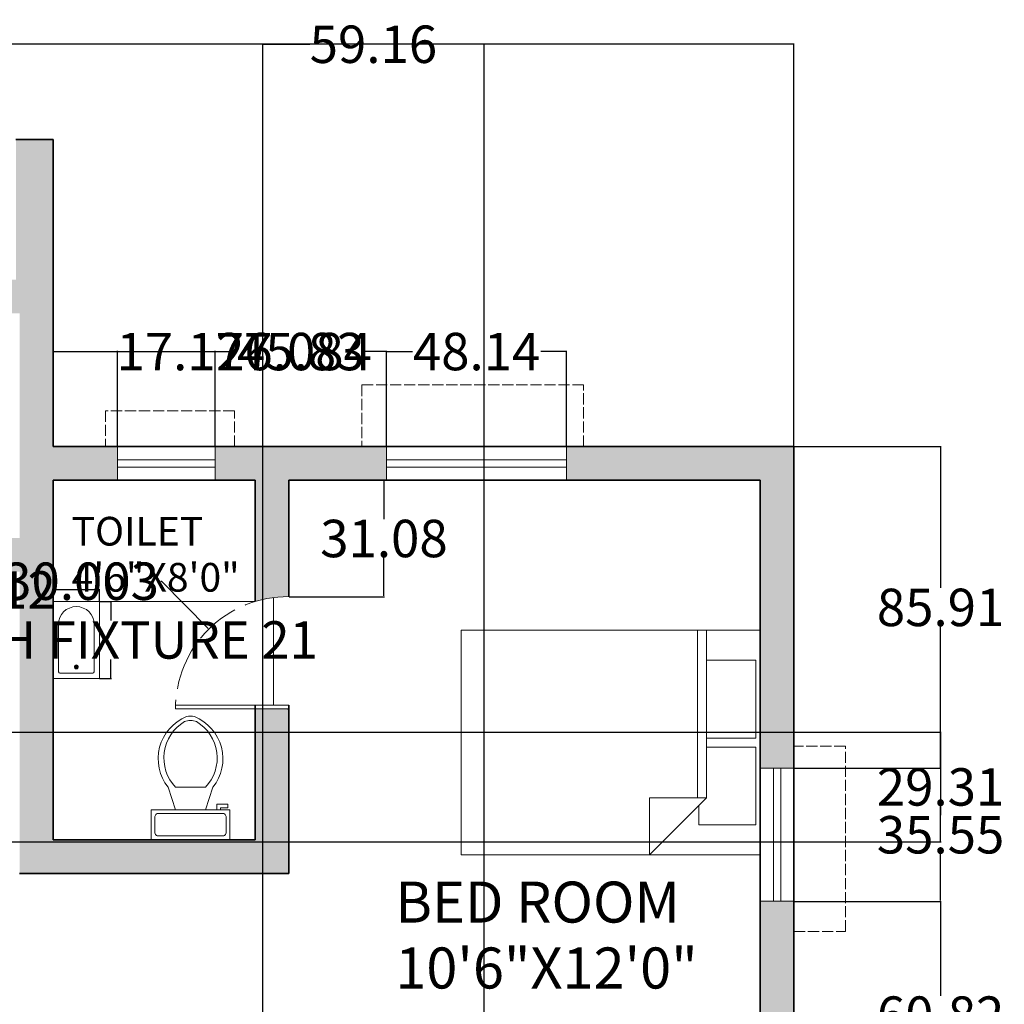
# Model space of a CAD drawing. Units: inches. Extents: x 143 to 746, y -392 to 145.
# Tile 6 of 6: x 473 to 736, y -118 to 145. Entities that reach past the tile are written whole.
import ezdxf

# ---------------------------------------------------------------- set-up
doc = ezdxf.new("R2010")
doc.units = ezdxf.units.IN
doc.header["$MEASUREMENT"] = 0
doc.linetypes.add('ACAD_ISO02W100', pattern=[15, 12, -3])
for name, color, linetype, lineweight in [('A-ANNO-DIMS', 2, 'Continuous', 18), ('A-AREA-IDEN', 7, 'Continuous', 20), ('A-DOOR', 3, 'Continuous', 18), ('A-DOOR-SWNG', 3, 'ACAD_ISO02W100', 13), ('A-FLOR-FIXT', 9, 'Continuous', 18), ('A-FURN', 8, 'Continuous', 18), ('A-GLAZ', 4, 'Continuous', 18), ('A-GLAZ-OVHD', 4, 'ACAD_ISO02W100', 13), ('A-WALL', 7, 'Continuous', 35)]:
    doc.layers.add(name, color=color, linetype=linetype, lineweight=lineweight)
doc.layers.add('A-WALL-PATT', color=252, linetype='Continuous', lineweight=13, true_color=0x939598)
doc.styles.get("Standard").update_dxf_attribs({"font": 'arial.ttf'})
doc.dimstyles.get("Standard").update_dxf_attribs({"dimtxt": 10, "dimasz": 0.18, "dimexe": 0.18, "dimexo": 0.0625, "dimgap": 0.09, "dimtad": 0, "dimtih": 1, "dimtoh": 1, "dimdec": 0, "dimzin": 0, "dimdsep": 46, "dimlunit": 3, "dimtxsty": 'Standard', "dimcen": 0.09, "dimadec": 0, "dimazin": 0, "dimtfac": 1, "dimtdec": 0, "dimtofl": 0, "dimtmove": 0, "dimatfit": 3, "dimfxl": 1, "dimtolj": 1, "dimtzin": 0, "dimarcsym": 0})

# ---------------------------------------------------------------- blocks, each defined once
blk = doc.blocks.new('Bath Tub - 26 x 60 in.')
for p, q in [((8, -18), (10, -18)), ((9, -17), (9, -19))]:
    blk.add_line(p, q)
blk.add_lwpolyline([(0, -36), (0, 0), (60, 0), (60, -36)], close=True)
for points in [[(4, -30), (4, -6)], [(6, -4), (42, -4)], [(42, -32), (6, -32)]]:
    blk.add_lwpolyline(points)
for radius in [1.5, 1]:
    blk.add_circle((9, -18), radius)
for centre, radius, start, end in [((5.75, -5.75), 1.77, 81.8699, 188.1301), ((42, -18), 14, 270, 90), ((5.75, -30.25), 1.77, 171.8699, 278.1301)]:
    blk.add_arc(centre, radius, start, end)
blk = doc.blocks.new('Toilet - top')
for p, q in [((9.5, -6), (9.5, -2)), ((-10, -8.5), (-8, -8.5)), ((-10, -9.5), (-10, -8.5)), ((-7, -9.5), (-10, -9.5)), ((-8, -8.5), (-8, -8)), ((-7, -8), (-7, -9.5)), ((-4, -8), (-6, -14)), ((4, -8), (6, -14)), ((4, -14), (-4, -14))]:
    blk.add_line(p, q)
blk.add_lwpolyline([(10.5, -8), (10.5, 0), (-10.5, 0), (-10.5, -8)], close=True)
for points in [[(-9.5, -2), (-9.5, -6)], [(8.5, -1), (-8.5, -1)], [(-8.5, -7), (8.5, -7)]]:
    blk.add_lwpolyline(points)
for centre, radius, start, end in [((-8.62, -1.88), 0.884, 81.8699, 188.1301), ((8.62, -1.88), 0.884, 351.8699, 98.1301), ((-8.62, -6.12), 0.884, 171.8699, 278.1301), ((8.62, -6.12), 0.884, 261.8699, 8.1301), ((3.52, -21.58), 12.17, 141.4691, 247.9714), ((4.2, -21.82), 11.33, 136.3677, 238.9468), ((-3.52, -21.58), 12.17, 292.0284, 38.5307), ((-4.2, -21.82), 11.33, 301.053, 43.6321), ((0, -27.88), 4, 245.7318, 294.2682), ((0, -29), 4, 254.8605, 285.1395)]:
    blk.add_arc(centre, radius, start, end)
blk = doc.blocks.new('Bed - Queen')
for p, q in [((0, -80.00003), (0, 0)), ((0, 0), (59.99999, 0)), ((59.99999, 0), (59.99999, -80.00003)), ((7.99999, -1.2), (28.79998, -1.2)), ((7.99999, -14.4), (7.99999, -1.2)), ((28.79998, -1.2), (28.79998, -14.4)), ((31.19999, -1.2), (51.99999, -1.2)), ((31.19999, -14.4), (31.19999, -1.2)), ((51.99999, -1.2), (51.99999, -16.4)), ((0, -14.4), (44.8, -14.4)), ((59.99999, -29.6), (44.8, -14.4)), ((44.8, -14.4), (44.8, -29.6)), ((44.8, -16.8), (0, -16.8)), ((51.99999, -16.4), (46.79936, -16.4)), ((44.8, -29.6), (59.99999, -29.6)), ((59.99999, -80.00003), (0, -80.00003))]:
    blk.add_line(p, q)
blk = doc.blocks.new('WINDOW-SHADE-49IN')
at = {"ltscale": 0.25}
for p, q in [((49.48, 13.79), (0, 13.79)), ((0, 13.79), (0, 0)), ((49.48, 0), (49.48, 13.79))]:
    blk.add_line(p, q, dxfattribs=at)
blk = doc.blocks.new('*D16')
at = {"layer": 'A-ANNO-DIMS', "color": 0, "lineweight": -2, "transparency": 16777216}
for p, q in [((493.94, -9.97), (497.14, -9.97)), ((496.96, -10.15), (496.96, -15.06)), ((496.96, -30.36), (496.96, -25.45)), ((493.94, -30.54), (497.14, -30.54))]:
    blk.add_line(p, q, dxfattribs=at)
at = {"layer": 'A-ANNO-DIMS', "color": 0, "transparency": 16777216}
for points in [[(496.93, -10.15), (496.99, -10.15), (496.96, -9.97)], [(496.93, -30.36), (496.99, -30.36), (496.96, -30.54)]]:
    blk.add_solid(points, dxfattribs=at)
at = {"layer": 'Defpoints', "color": 0, "transparency": 16777216}
for p in [(493.88, -9.97), (496.96, -9.97), (493.88, -30.54)]:
    blk.add_point(p, dxfattribs=at)
at = {"layer": 'A-ANNO-DIMS', "color": 0, "transparency": 16777216, "insert": (496.96, -20.25), "char_height": 10, "attachment_point": 5}
blk.add_mtext('\\A1;BATH FIXTURE 21', dxfattribs=at)
blk = doc.blocks.new('*D17')
at = {"layer": 'A-ANNO-DIMS', "color": 0, "lineweight": -2, "transparency": 16777216}
for p, q in [((481.54, -6.88), (481.36, -6.88)), ((481.54, -9.91), (481.54, -6.7)), ((493.7, -6.88), (481.72, -6.88)), ((493.88, -9.91), (493.88, -6.7))]:
    blk.add_line(p, q, dxfattribs=at)
at = {"layer": 'A-ANNO-DIMS', "color": 0, "transparency": 16777216}
for points in [[(481.72, -6.85), (481.72, -6.91), (481.54, -6.88)], [(493.7, -6.85), (493.7, -6.91), (493.88, -6.88)]]:
    blk.add_solid(points, dxfattribs=at)
at = {"layer": 'Defpoints', "color": 0, "transparency": 16777216}
for p in [(481.54, -6.88), (481.54, -9.97), (493.88, -9.97)]:
    blk.add_point(p, dxfattribs=at)
at = {"layer": 'A-ANNO-DIMS', "color": 0, "transparency": 16777216, "insert": (474.63, -6.88), "char_height": 10, "attachment_point": 5}
blk.add_mtext('\\A1;12', dxfattribs=at)
blk = doc.blocks.new('*D43')
at = {"layer": 'A-ANNO-DIMS', "color": 0, "lineweight": -2, "transparency": 16777216}
for p, q in [((189.54, 28.45), (189.54, 139.06)), ((189.72, 138.88), (423.22, 138.88)), ((679.36, 138.88), (445.86, 138.88)), ((679.54, 31.45), (679.54, 139.06))]:
    blk.add_line(p, q, dxfattribs=at)
at = {"layer": 'A-ANNO-DIMS', "color": 0, "transparency": 16777216}
for points in [[(189.72, 138.91), (189.72, 138.85), (189.54, 138.88)], [(679.36, 138.91), (679.36, 138.85), (679.54, 138.88)]]:
    blk.add_solid(points, dxfattribs=at)
at = {"layer": 'Defpoints', "color": 0, "transparency": 16777216}
for p in [(679.54, 138.88), (679.54, 31.39), (189.54, 28.39)]:
    blk.add_point(p, dxfattribs=at)
at = {"layer": 'A-ANNO-DIMS', "color": 0, "transparency": 16777216, "insert": (434.54, 138.88), "char_height": 10, "attachment_point": 5}
blk.add_mtext('\\A1;490', dxfattribs=at)
blk = doc.blocks.new('*D53')
at = {"layer": 'A-ANNO-DIMS', "color": 0, "lineweight": -2, "transparency": 16777216}
for p, q in [((481.54, 31.45), (481.54, 56.97)), ((481.72, 56.79), (498.53, 56.79)), ((498.71, 31.45), (498.71, 56.97)), ((498.71, 56.79), (498.89, 56.79))]:
    blk.add_line(p, q, dxfattribs=at)
at = {"layer": 'A-ANNO-DIMS', "color": 0, "transparency": 16777216}
for points in [[(481.72, 56.82), (481.72, 56.76), (481.54, 56.79)], [(498.53, 56.82), (498.53, 56.76), (498.71, 56.79)]]:
    blk.add_solid(points, dxfattribs=at)
at = {"layer": 'Defpoints', "color": 0, "transparency": 16777216}
for p in [(498.71, 56.79), (481.54, 31.39), (498.71, 31.39)]:
    blk.add_point(p, dxfattribs=at)
at = {"layer": 'A-ANNO-DIMS', "color": 0, "transparency": 16777216, "insert": (519.27, 56.79), "char_height": 10, "attachment_point": 5}
blk.add_mtext('\\A1;17.177', dxfattribs=at)
blk = doc.blocks.new('*D54')
at = {"layer": 'A-ANNO-DIMS', "color": 0, "lineweight": -2, "transparency": 16777216}
for p, q in [((498.71, 31.45), (498.71, 56.97)), ((498.89, 56.79), (524.62, 56.79)), ((524.8, 31.45), (524.8, 56.97)), ((524.8, 56.79), (524.98, 56.79))]:
    blk.add_line(p, q, dxfattribs=at)
at = {"layer": 'A-ANNO-DIMS', "color": 0, "transparency": 16777216}
for points in [[(498.89, 56.82), (498.89, 56.76), (498.71, 56.79)], [(524.62, 56.82), (524.62, 56.76), (524.8, 56.79)]]:
    blk.add_solid(points, dxfattribs=at)
at = {"layer": 'Defpoints', "color": 0, "transparency": 16777216}
for p in [(524.8, 56.79), (498.71, 31.39), (524.8, 31.39)]:
    blk.add_point(p, dxfattribs=at)
at = {"layer": 'A-ANNO-DIMS', "color": 0, "transparency": 16777216, "insert": (545.89, 56.79), "char_height": 10, "attachment_point": 5}
blk.add_mtext('\\A1;26.084', dxfattribs=at)
blk = doc.blocks.new('*D55')
at = {"layer": 'A-ANNO-DIMS', "color": 0, "lineweight": -2, "transparency": 16777216}
for p, q in [((524.8, 31.45), (524.8, 56.97)), ((524.98, 56.79), (530.55, 56.79)), ((570.45, 56.79), (564.88, 56.79)), ((570.63, 31.45), (570.63, 56.97))]:
    blk.add_line(p, q, dxfattribs=at)
at = {"layer": 'A-ANNO-DIMS', "color": 0, "transparency": 16777216}
for points in [[(524.98, 56.82), (524.98, 56.76), (524.8, 56.79)], [(570.45, 56.82), (570.45, 56.76), (570.63, 56.79)]]:
    blk.add_solid(points, dxfattribs=at)
at = {"layer": 'Defpoints', "color": 0, "transparency": 16777216}
for p in [(570.63, 56.79), (524.8, 31.39), (570.63, 31.39)]:
    blk.add_point(p, dxfattribs=at)
at = {"layer": 'A-ANNO-DIMS', "color": 0, "transparency": 16777216, "insert": (547.71, 56.79), "char_height": 10, "attachment_point": 5}
blk.add_mtext('\\A1;45.83', dxfattribs=at)
blk = doc.blocks.new('*D56')
at = {"layer": 'A-ANNO-DIMS', "color": 0, "lineweight": -2, "transparency": 16777216}
for p, q in [((570.63, 31.45), (570.63, 56.97)), ((570.81, 56.79), (577.56, 56.79)), ((618.59, 56.79), (611.84, 56.79)), ((618.77, 31.45), (618.77, 56.97))]:
    blk.add_line(p, q, dxfattribs=at)
at = {"layer": 'A-ANNO-DIMS', "color": 0, "transparency": 16777216}
for points in [[(570.81, 56.82), (570.81, 56.76), (570.63, 56.79)], [(618.59, 56.82), (618.59, 56.76), (618.77, 56.79)]]:
    blk.add_solid(points, dxfattribs=at)
at = {"layer": 'Defpoints', "color": 0, "transparency": 16777216}
for p in [(618.77, 56.79), (570.63, 31.39), (618.77, 31.39)]:
    blk.add_point(p, dxfattribs=at)
at = {"layer": 'A-ANNO-DIMS', "color": 0, "transparency": 16777216, "insert": (594.7, 56.79), "char_height": 10, "attachment_point": 5}
blk.add_mtext('\\A1;48.14', dxfattribs=at)
blk = doc.blocks.new('*D57')
at = {"layer": 'A-ANNO-DIMS', "color": 0, "lineweight": -2, "transparency": 16777216}
for p, q in [((679.6, 31.39), (718.91, 31.39)), ((718.73, 31.21), (718.73, -6.37)), ((718.73, -54.34), (718.73, -16.76)), ((679.6, -54.52), (718.91, -54.52))]:
    blk.add_line(p, q, dxfattribs=at)
at = {"layer": 'A-ANNO-DIMS', "color": 0, "transparency": 16777216}
for points in [[(718.7, 31.21), (718.76, 31.21), (718.73, 31.39)], [(718.7, -54.34), (718.76, -54.34), (718.73, -54.52)]]:
    blk.add_solid(points, dxfattribs=at)
at = {"layer": 'Defpoints', "color": 0, "transparency": 16777216}
for p in [(679.54, 31.39), (679.54, -54.52), (718.73, -54.52)]:
    blk.add_point(p, dxfattribs=at)
at = {"layer": 'A-ANNO-DIMS', "color": 0, "transparency": 16777216, "insert": (718.73, -11.56), "char_height": 10, "attachment_point": 5}
blk.add_mtext('\\A1;85.91', dxfattribs=at)
blk = doc.blocks.new('*D58')
at = {"layer": 'A-ANNO-DIMS', "color": 0, "lineweight": -2, "transparency": 16777216}
for p, q in [((679.6, -54.52), (718.91, -54.52)), ((718.73, -54.7), (718.73, -67.1)), ((718.73, -89.9), (718.73, -77.5)), ((679.6, -90.08), (718.91, -90.08))]:
    blk.add_line(p, q, dxfattribs=at)
at = {"layer": 'A-ANNO-DIMS', "color": 0, "transparency": 16777216}
for points in [[(718.7, -54.7), (718.76, -54.7), (718.73, -54.52)], [(718.7, -89.9), (718.76, -89.9), (718.73, -90.08)]]:
    blk.add_solid(points, dxfattribs=at)
at = {"layer": 'Defpoints', "color": 0, "transparency": 16777216}
for p in [(679.54, -54.52), (679.54, -90.08), (718.73, -90.08)]:
    blk.add_point(p, dxfattribs=at)
at = {"layer": 'A-ANNO-DIMS', "color": 0, "transparency": 16777216, "insert": (718.73, -72.3), "char_height": 10, "attachment_point": 5}
blk.add_mtext('\\A1;35.55', dxfattribs=at)
blk = doc.blocks.new('*D59')
at = {"layer": 'A-ANNO-DIMS', "color": 0, "lineweight": -2, "transparency": 16777216}
for p, q in [((679.6, -90.08), (718.91, -90.08)), ((718.73, -90.26), (718.73, -115.29)), ((718.73, -150.71), (718.73, -125.68)), ((679.6, -150.89), (718.91, -150.89))]:
    blk.add_line(p, q, dxfattribs=at)
at = {"layer": 'A-ANNO-DIMS', "color": 0, "transparency": 16777216}
for points in [[(718.7, -90.26), (718.76, -90.26), (718.73, -90.08)], [(718.7, -150.71), (718.76, -150.71), (718.73, -150.89)]]:
    blk.add_solid(points, dxfattribs=at)
at = {"layer": 'Defpoints', "color": 0, "transparency": 16777216}
for p in [(679.54, -90.08), (679.54, -150.89), (718.73, -150.89)]:
    blk.add_point(p, dxfattribs=at)
at = {"layer": 'A-ANNO-DIMS', "color": 0, "transparency": 16777216, "insert": (718.73, -120.48), "char_height": 10, "attachment_point": 5}
blk.add_mtext('\\A1;60.82', dxfattribs=at)
blk = doc.blocks.new('*D65')
at = {"layer": 'A-ANNO-DIMS', "color": 0, "lineweight": -2, "transparency": 16777216}
for p, q in [((537.54, -212.72), (537.54, 139.06)), ((537.72, 138.88), (550.16, 138.88)), ((596.51, 138.88), (584.08, 138.88)), ((596.69, -212.72), (596.69, 139.06))]:
    blk.add_line(p, q, dxfattribs=at)
at = {"layer": 'A-ANNO-DIMS', "color": 0, "transparency": 16777216}
for points in [[(537.72, 138.91), (537.72, 138.85), (537.54, 138.88)], [(596.51, 138.91), (596.51, 138.85), (596.69, 138.88)]]:
    blk.add_solid(points, dxfattribs=at)
at = {"layer": 'Defpoints', "color": 0, "transparency": 16777216}
for p in [(596.69, 138.88), (537.54, -212.78), (596.69, -212.78)]:
    blk.add_point(p, dxfattribs=at)
at = {"layer": 'A-ANNO-DIMS', "color": 0, "transparency": 16777216, "insert": (567.12, 138.88), "char_height": 10, "attachment_point": 5}
blk.add_mtext('\\A1;59.16', dxfattribs=at)
blk = doc.blocks.new('*D69')
at = {"layer": 'A-ANNO-DIMS', "color": 0, "lineweight": -2, "transparency": 16777216}
for p, q in [((284.99, -44.86), (718.91, -44.86)), ((718.73, -45.04), (718.73, -54.32)), ((718.73, -73.99), (718.73, -64.72)), ((284.99, -74.17), (718.91, -74.17))]:
    blk.add_line(p, q, dxfattribs=at)
at = {"layer": 'A-ANNO-DIMS', "color": 0, "transparency": 16777216}
for points in [[(718.7, -45.04), (718.76, -45.04), (718.73, -44.86)], [(718.7, -73.99), (718.76, -73.99), (718.73, -74.17)]]:
    blk.add_solid(points, dxfattribs=at)
at = {"layer": 'Defpoints', "color": 0, "transparency": 16777216}
for p in [(284.93, -44.86), (284.93, -74.17), (718.73, -74.17)]:
    blk.add_point(p, dxfattribs=at)
at = {"layer": 'A-ANNO-DIMS', "color": 0, "transparency": 16777216, "insert": (718.73, -59.52), "char_height": 10, "attachment_point": 5}
blk.add_mtext('\\A1;29.31', dxfattribs=at)
blk = doc.blocks.new('*D71')
at = {"layer": 'A-ANNO-DIMS', "color": 0, "lineweight": -2, "transparency": 16777216}
for p, q in [((544.6, 22.39), (570.12, 22.39)), ((569.94, 22.21), (569.94, 12.05)), ((569.94, -8.51), (569.94, 1.65)), ((544.6, -8.69), (570.12, -8.69))]:
    blk.add_line(p, q, dxfattribs=at)
at = {"layer": 'A-ANNO-DIMS', "color": 0, "transparency": 16777216}
for points in [[(569.91, 22.21), (569.97, 22.21), (569.94, 22.39)], [(569.91, -8.51), (569.97, -8.51), (569.94, -8.69)]]:
    blk.add_solid(points, dxfattribs=at)
at = {"layer": 'Defpoints', "color": 0, "transparency": 16777216}
for p in [(544.54, 22.39), (544.54, -8.69), (569.94, -8.69)]:
    blk.add_point(p, dxfattribs=at)
at = {"layer": 'A-ANNO-DIMS', "color": 0, "transparency": 16777216, "insert": (569.94, 6.85), "char_height": 10, "attachment_point": 5}
blk.add_mtext('\\A1;31.08', dxfattribs=at)
blk = doc.blocks.new('*D79')
at = {"layer": 'A-ANNO-DIMS', "color": 0, "lineweight": -2, "transparency": 16777216}
for p, q in [((510.28, -4.57), (510.46, -4.57)), ((510.46, -4.57), (522.99, -17.23)), ((544.13, -38.69), (544.31, -38.69)), ((544.22, -38.78), (544.22, -38.6))]:
    blk.add_line(p, q, dxfattribs=at)
at = {"layer": 'A-ANNO-DIMS', "color": 0, "transparency": 16777216}
blk.add_solid([(523.01, -17.21), (522.97, -17.25), (523.12, -17.36)], dxfattribs=at)
at = {"layer": 'Defpoints', "color": 0, "transparency": 16777216}
for p in [(523.12, -17.36), (544.22, -38.69)]:
    blk.add_point(p, dxfattribs=at)
at = {"layer": 'A-ANNO-DIMS', "color": 0, "transparency": 16777216, "insert": (484.64, -4.57), "char_height": 10, "attachment_point": 5}
blk.add_mtext('\\A1;R30.003', dxfattribs=at)

msp = doc.modelspace()

# ---------------------------------------------------------------- hatches: boundary and pattern name
at = {"layer": 'A-WALL-PATT'}
h = msp.add_hatch(color=256, dxfattribs=at)
h.dxf.hatch_style = 1
h.paths.add_polyline_path([(198.538, 19.3924), (257.4275, 19.3924), (257.4275, 28.3924), (189.538, 28.3924), (189.538, -95.6731, -0.06325422), (198.538, -96.8162)])
h.paths.add_polyline_path([(339.538, 66.969), (471.538, 66.969), (472.538, 66.969), (472.538, 31.3924), (472.538, 6.969), (451.2296, 6.969), (451.2296, -2.031), (472.538, -2.031), (472.538, -82.6076), (544.538, -82.6076), (544.538, -38.6894), (535.538, -38.6894), (535.538, -73.6076), (481.538, -73.6076), (481.538, 22.3924), (498.7149, 22.3924), (498.7149, 31.3924), (481.538, 31.3924), (481.538, 66.969), (481.538, 113.4779), (471.538, 113.4779), (471.538, 75.969), (339.538, 75.969), (339.538, 113.4779), (330.538, 113.4779), (330.538, 66.969), (330.538, 28.3924), (293.6446, 28.3924), (293.6446, 19.3924), (330.538, 19.3924), (330.538, 6.969), (330.538, -2.031), (364.5099, -2.031), (364.5099, 6.969), (339.538, 6.969)])
h.paths.add_polyline_path([(570.63, 31.3924), (544.538, 31.3924), (524.7988, 31.3924), (524.7988, 22.3924), (535.538, 22.3924), (535.538, -9.9696, -0.0761882), (544.538, -8.6878), (544.538, 22.3924), (570.63, 22.3924)])
h.paths.add_polyline_path([(679.538, 31.3924), (618.768, 31.3924), (618.768, 22.3924), (670.538, 22.3924), (670.538, -54.5218), (679.538, -54.5218)])
h.paths.add_polyline_path([(679.538, -90.0753), (670.538, -90.0753), (670.538, -121.6076), (537.538, -121.6076), (528.538, -121.6076), (528.538, -130.6076), (537.538, -130.6076), (670.538, -130.6076), (670.538, -150.8923), (679.538, -150.8923)])
h.paths.add_polyline_path([(679.538, -187.0502), (670.538, -187.0502), (670.538, -232.6076), (636.538, -232.6076, -0.07632083), (635.1562, -241.6076), (670.538, -241.6076), (670.538, -256.599), (679.538, -256.599)])
h.paths.add_polyline_path([(606.538, -232.6076), (537.538, -232.6076), (537.538, -241.6076), (597.538, -241.6076), (597.538, -337.6076), (590.545, -337.6076), (590.545, -346.6076), (679.538, -346.6076), (679.538, -316.1251), (670.538, -316.1251), (670.538, -337.6076), (606.538, -337.6076)])
h.paths.add_polyline_path([(537.538, -181.6076), (537.538, -172.6076), (528.538, -172.6076), (528.538, -209.005), (528.538, -269.6672, -0.07632083), (537.538, -271.0491)])
h.paths.add_polyline_path([(566.8252, -337.6076), (537.538, -337.6076), (537.538, -299.6672), (528.538, -299.6672), (528.538, -337.6076), (513.484, -337.6076), (513.484, -346.6076), (566.8252, -346.6076)])
h.paths.add_polyline_path([(477.1278, -337.6076), (408.538, -337.6076), (408.538, -229.6076), (408.538, -181.6076), (493.5793, -181.6076, -0.06316411), (492.538, -172.6076), (399.538, -172.6076), (399.538, -229.6076), (399.538, -337.6076), (388.659, -337.6076), (388.659, -346.6076), (477.1278, -346.6076)])
h.paths.add_polyline_path([(364.4504, -337.6076), (339.538, -337.6076), (339.538, -301.3371), (330.538, -301.3371), (330.538, -337.6076), (307.2736, -337.6076), (307.2736, -346.6076), (364.4504, -346.6076)])
h.paths.add_polyline_path([(339.538, -229.6076), (399.538, -229.6076), (399.538, -220.6076), (369.1898, -220.6076), (330.538, -220.6076), (330.538, -271.2389, -0.07612824), (339.538, -272.6672)])
h.paths.add_polyline_path([(271.3704, -337.6076), (198.538, -337.6076), (198.538, -181.6076), (339.538, -181.6076), (339.538, -172.6076), (198.538, -172.6076), (198.538, -131.6731), (189.538, -131.6731), (189.538, -346.6076), (271.3704, -346.6076)])

# ---------------------------------------------------------------- linework, layer by layer
at = {"layer": 'A-DOOR'}
for p, q in [((540.3705, -37.6894), (540.3793, -8.9329)), ((544.538, -37.6894), (514.2163, -37.6894)), ((544.538, -38.6894), (514.2163, -38.6894)), ((544.538, -38.6894), (544.538, -37.6894))]:
    msp.add_line(p, q, dxfattribs=at)
at = {"layer": 'A-DOOR-SWNG'}
msp.add_arc((544.2196, -38.6894), 30.0033, 89.3919, 180, dxfattribs=at)
at = {"layer": 'A-FLOR-FIXT'}
msp.add_line((535.538, -9.9696), (481.538, -9.9696), dxfattribs=at)
at = {"layer": 'A-GLAZ'}
for p, q in [((498.7149, 31.3924), (498.7149, 22.3924)), ((524.7988, 31.3924), (524.7988, 22.3924)), ((570.63, 31.3924), (570.63, 22.3924)), ((618.768, 26.8924), (618.768, 31.3924)), ((618.768, 31.3924), (618.768, 22.3924)), ((498.7149, 27.8924), (524.7988, 27.8924)), ((570.63, 27.8924), (618.768, 27.8924)), ((498.7149, 25.8924), (524.7988, 25.8924)), ((570.63, 25.8924), (618.768, 25.8924)), ((675.038, -54.5218), (670.538, -54.5218)), ((670.538, -54.5218), (679.538, -54.5218)), ((674.038, -90.0753), (674.038, -54.5218)), ((676.038, -90.0753), (676.038, -54.5218)), ((670.538, -90.0753), (679.538, -90.0753))]:
    msp.add_line(p, q, dxfattribs=at)
at = {"layer": 'A-GLAZ-OVHD', "ltscale": 0.25}
for p, q in [((623.3201, 47.9098), (564.0433, 47.9098)), ((564.0433, 47.9098), (564.0433, 31.3924)), ((623.3201, 31.3924), (623.3201, 47.9098)), ((529.9606, 40.9855), (495.5336, 40.9855)), ((495.5336, 40.9855), (495.5336, 31.3924)), ((529.9606, 31.3924), (529.9606, 40.9855))]:
    msp.add_line(p, q, dxfattribs=at)
at = {"layer": 'A-WALL'}
for p, q in [((471.538, 113.4779), (481.538, 113.4779)), ((481.538, 113.4779), (481.538, 66.969)), ((481.538, 66.969), (481.538, 31.3924)), ((481.538, 31.3924), (544.538, 31.3924)), ((679.538, 31.3924), (544.538, 31.3924)), ((679.538, -346.6076), (679.538, 31.3924)), ((481.538, 22.3924), (535.538, 22.3924)), ((481.538, -73.6076), (481.538, 22.3924)), ((535.538, 22.3924), (535.538, -9.9696)), ((670.538, 22.3924), (544.538, 22.3924)), ((544.538, 22.3924), (544.538, -8.6878)), ((670.538, -121.6076), (670.538, 22.3924)), ((535.538, -37.6894), (535.538, -73.6076)), ((544.538, -37.6894), (544.538, -82.6076)), ((535.538, -73.6076), (481.538, -73.6076)), ((544.538, -82.6076), (472.538, -82.6076))]:
    msp.add_line(p, q, dxfattribs=at)

# ---------------------------------------------------------------- block references
at = {"layer": 'A-FLOR-FIXT', "xscale": 0.3427904790576684, "yscale": 0.3427904790576684, "zscale": 0.3427904790576684, "rotation": 90}
msp.add_blockref('Bath Tub - 26 x 60 in.', (481.538, -30.5371), dxfattribs=at)
at = {"layer": 'A-FLOR-FIXT', "rotation": 180}
msp.add_blockref('Toilet - top', (518.2309, -73.6076), dxfattribs=at)
at = {"layer": 'A-FURN', "rotation": 270}
msp.add_blockref('Bed - Queen', (670.538, -17.6588), dxfattribs=at)
at = {"layer": 'A-GLAZ-OVHD', "rotation": 270}
msp.add_blockref('WINDOW-SHADE-49IN', (679.5376, -48.6184), dxfattribs=at)

# ---------------------------------------------------------------- texts
at = {"layer": 'A-AREA-IDEN'}
for s, height, p in [('TOILET', 7.66535, (486.4492, 4.9646)), ('4\'6"X8\'0"', 7.66535, (486.4492, -7.3491)), ('BED ROOM', 10.95807, (572.97, -95.7629)), ('10\'6"X12\'0"', 10.958074, (572.97, -113.3661))]:
    msp.add_text(s, height=height, dxfattribs=at).set_placement(p)

# ---------------------------------------------------------------- dimensions: what is measured, and where the dimension line sits
at = {"layer": 'A-ANNO-DIMS'}
for base, p1, p2, override, picture, middle in [((679.538, 138.8779), (189.538, 28.3924), (679.538, 31.3924), {"dimdec": 0, "dimlfac": 1, "dimrnd": 0, "dimzin": 0, "dimdsep": 46, "dimlunit": 2}, '*D43', (434.538, 138.8779)), ((596.695, 138.8779), (537.538, -212.7788), (596.695, -212.7788), {"dimdec": 2, "dimlfac": 1, "dimrnd": 0, "dimzin": 0, "dimdsep": 46, "dimlunit": 2}, '*D65', (567.1165, 138.8779)), ((498.7149, 56.7924), (481.538, 31.3924), (498.7149, 31.3924), {"dimdec": 3, "dimlfac": 1, "dimrnd": 0, "dimzin": 0, "dimdsep": 46, "dimlunit": 2}, '*D53', (519.2714, 56.7924)), ((524.7988, 56.7924), (498.7149, 31.3924), (524.7988, 31.3924), {"dimdec": 3, "dimlfac": 1, "dimrnd": 0, "dimzin": 0, "dimdsep": 46, "dimlunit": 2}, '*D54', (545.8908, 56.7924)), ((570.63, 56.7924), (524.7988, 31.3924), (570.63, 31.3924), {"dimdec": 2, "dimlfac": 1, "dimrnd": 0, "dimzin": 0, "dimdsep": 46, "dimlunit": 2}, '*D55', (547.7144, 56.7924)), ((618.768, 56.7924), (570.63, 31.3924), (618.768, 31.3924), {"dimdec": 2, "dimlfac": 1, "dimrnd": 0, "dimzin": 0, "dimdsep": 46, "dimlunit": 2}, '*D56', (594.699, 56.7924))]:
    dim = msp.add_linear_dim(base=base, p1=p1, p2=p2, dimstyle='Standard', override=override, dxfattribs=at)
    dim.commit()
    dim.dimension.update_dxf_attribs({"geometry": picture, "text_midpoint": middle})
for base, p1, p2, angle, override, picture, middle in [((718.7255, -54.5218), (679.538, 31.3924), (679.538, -54.5218), 90, {"dimdec": 2, "dimlfac": 1, "dimrnd": 0, "dimzin": 0, "dimdsep": 46, "dimlunit": 2}, '*D57', (718.7255, -11.5647)), ((569.938, -8.6878), (544.538, 22.3924), (544.538, -8.6878), 270, {"dimdec": 2, "dimlfac": 1, "dimrnd": 0, "dimzin": 0, "dimdsep": 46, "dimlunit": 2}, '*D71', (569.938, 6.8523)), ((481.538, -6.8845), (493.8785, -9.9696), (481.538, -9.9696), 180, {"dimdec": 0, "dimlfac": 1, "dimrnd": 0, "dimzin": 0, "dimdsep": 46, "dimlunit": 2}, '*D17', (474.6275, -6.8845)), ((718.7255, -74.1707), (284.9288, -44.8632), (284.9288, -74.1707), 90, {"dimdec": 2, "dimlfac": 1, "dimrnd": 0, "dimzin": 0, "dimdsep": 46, "dimlunit": 2}, '*D69', (718.7255, -59.5169)), ((718.7255, -90.0753), (679.538, -54.5218), (679.538, -90.0753), 90, {"dimdec": 2, "dimlfac": 1, "dimrnd": 0, "dimzin": 0, "dimdsep": 46, "dimlunit": 2}, '*D58', (718.7255, -72.2985)), ((718.7255, -150.8923), (679.538, -90.0753), (679.538, -150.8923), 90, {"dimdec": 2, "dimlfac": 1, "dimrnd": 0, "dimzin": 0, "dimdsep": 46, "dimlunit": 2}, '*D59', (718.7255, -120.4838))]:
    dim = msp.add_linear_dim(base=base, p1=p1, p2=p2, angle=angle, dimstyle='Standard', override=override, dxfattribs=at)
    dim.commit()
    dim.dimension.update_dxf_attribs({"geometry": picture, "text_midpoint": middle})
dim = msp.add_linear_dim(base=(496.9636, -9.9696), p1=(493.8785, -30.5371), p2=(493.8785, -9.9696), angle=90, text='BATH FIXTURE <>', dimstyle='Standard', override={"dimdec": 0, "dimlfac": 1, "dimrnd": 0, "dimzin": 0, "dimdsep": 46, "dimlunit": 2}, dxfattribs=at)
dim.commit()
dim.dimension.update_dxf_attribs({"geometry": '*D16', "text_midpoint": (496.9636, -20.2533)})
dim = msp.add_radius_dim(center=(544.2196, -38.6894), mpoint=(523.1168, -17.3618), dimstyle='Standard', override={"dimdec": 3, "dimlfac": 1, "dimrnd": 0, "dimzin": 0, "dimdsep": 46, "dimlunit": 2}, dxfattribs=at)
dim.commit()
dim.dimension.update_dxf_attribs({"geometry": '*D79', "text_midpoint": (484.6428, -4.5652), "dimtype": 164})

doc.saveas('drawing.dxf')
